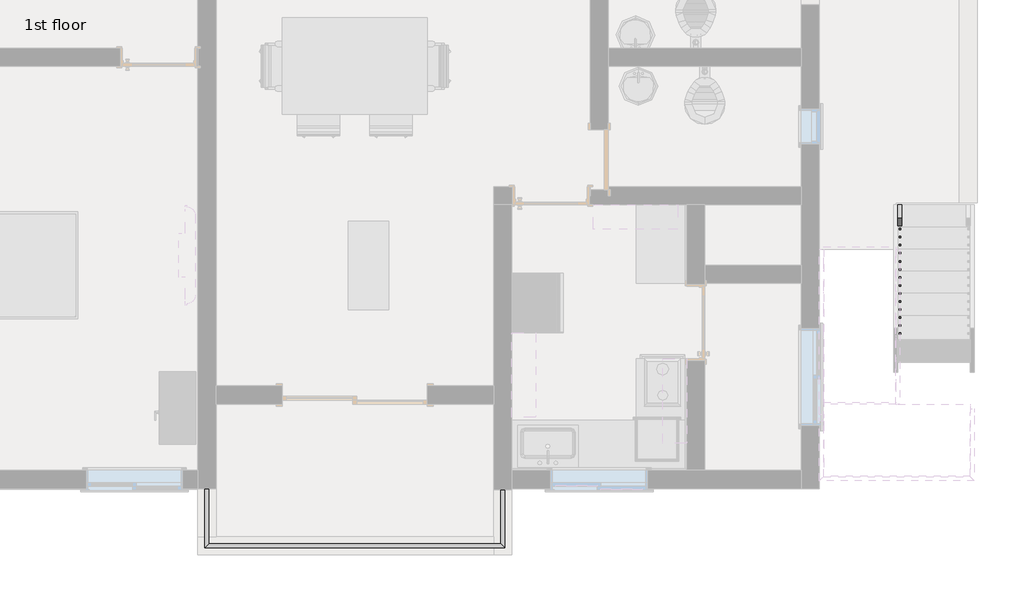
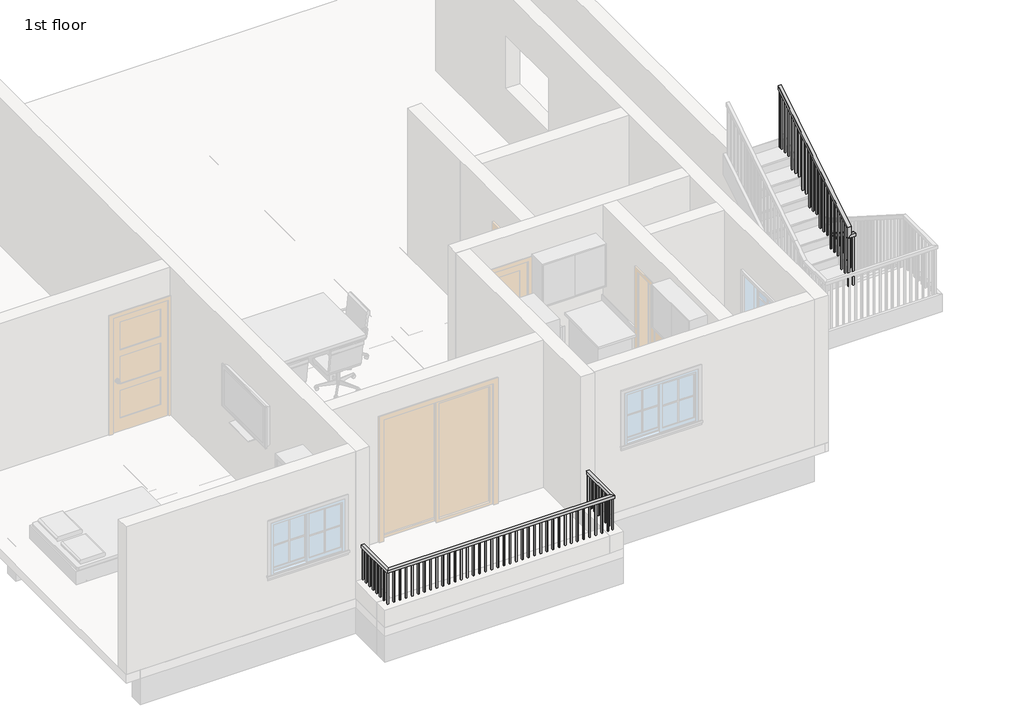
# One storey, part 4 of 8: 2 railings.
"""IFC4 building model written with IfcOpenShell, lengths in millimetres."""

from ifc_helpers import new_model, si_unit, frame, origin, place, context, project, spatial, polyline, outline, extrude, faceted_brep, element, save

model = new_model("IFC4")

# Units and contexts
model_context = context("Model", 3, world=origin())
ifc_project = project(units=[si_unit("LENGTHUNIT", "METRE", prefix="MILLI")], contexts=[model_context])

# Site, building, storey
site = spatial("IfcSite", under=ifc_project)
building = spatial("IfcBuilding", under=site)
storey = spatial("IfcBuildingStorey", under=building, Name="1st floor", Elevation=3810.0)

# Railings
placement = place(None, origin())
element("IfcRailing", 1, ObjectType="Handrail - Rectangular", at=placement, inside=storey, context=model_context, shape_type="SolidModel", body=[
    faceted_brep([(-12350.8993763, -4611.6564015, 4724.4), (-12350.8993763, -4611.6564015, 4673.6), (-12401.6993763, -4611.6564015, 4673.6), (-12401.6993763, -4611.6564015, 4724.4), (-12350.8993763, -5303.8064015, 4724.4), (-12350.8993763, -5303.8064015, 4673.6), (-12401.6993763, -5354.6064015, 4673.6), (-12401.6993763, -5354.6064015, 4724.4), (-8667.8993763, -5303.8064015, 4724.4), (-8667.8993763, -5303.8064015, 4673.6), (-8617.0993763, -5354.6064015, 4673.6), (-8617.0993763, -5354.6064015, 4724.4), (-8667.8993763, -4618.0064015, 4724.4), (-8617.0993763, -4618.0064015, 4724.4), (-8617.0993763, -4618.0064015, 4673.6), (-8667.8993763, -4618.0064015, 4673.6)], [[[0, 1, 2, 3]], [[1, 0, 4, 5]], [[2, 1, 5, 6]], [[3, 2, 6, 7]], [[0, 3, 7, 4]], [[5, 4, 8, 9]], [[6, 5, 9, 10]], [[7, 6, 10, 11]], [[4, 7, 11, 8]], [[12, 13, 14, 15]], [[9, 8, 12, 15]], [[10, 9, 15, 14]], [[11, 10, 14, 13]], [[8, 11, 13, 12]]]),
    extrude(outline(polyline([(-8632.9743763, -4729.1314015), (-8652.0243763, -4729.1314015), (-8652.0243763, -4710.0814015), (-8632.9743763, -4710.0814015), (-8632.9743763, -4729.1314015)])), frame((0.0, 0.0, 3810.0), z_axis=(0.0, 0.0, 1.0), x_axis=(1.0, 0.0, 0.0)), (0.0, 0.0, 1.0), 863.6),
    extrude(outline(polyline([(-8632.9743763, -4830.7314015), (-8652.0243763, -4830.7314015), (-8652.0243763, -4811.6814015), (-8632.9743763, -4811.6814015), (-8632.9743763, -4830.7314015)])), frame((0.0, 0.0, 3810.0), z_axis=(0.0, 0.0, 1.0), x_axis=(1.0, 0.0, 0.0)), (0.0, 0.0, 1.0), 863.6),
    extrude(outline(polyline([(-8632.9743763, -4932.3314015), (-8652.0243763, -4932.3314015), (-8652.0243763, -4913.2814015), (-8632.9743763, -4913.2814015), (-8632.9743763, -4932.3314015)])), frame((0.0, 0.0, 3810.0), z_axis=(0.0, 0.0, 1.0), x_axis=(1.0, 0.0, 0.0)), (0.0, 0.0, 1.0), 863.6),
    extrude(outline(polyline([(-8632.9743763, -5033.9314015), (-8652.0243763, -5033.9314015), (-8652.0243763, -5014.8814015), (-8632.9743763, -5014.8814015), (-8632.9743763, -5033.9314015)])), frame((0.0, 0.0, 3810.0), z_axis=(0.0, 0.0, 1.0), x_axis=(1.0, 0.0, 0.0)), (0.0, 0.0, 1.0), 863.6),
    extrude(outline(polyline([(-8632.9743763, -5135.5314015), (-8652.0243763, -5135.5314015), (-8652.0243763, -5116.4814015), (-8632.9743763, -5116.4814015), (-8632.9743763, -5135.5314015)])), frame((0.0, 0.0, 3810.0), z_axis=(0.0, 0.0, 1.0), x_axis=(1.0, 0.0, 0.0)), (0.0, 0.0, 1.0), 863.6),
    extrude(outline(polyline([(-8632.9743763, -5237.1314015), (-8652.0243763, -5237.1314015), (-8652.0243763, -5218.0814015), (-8632.9743763, -5218.0814015), (-8632.9743763, -5237.1314015)])), frame((0.0, 0.0, 3810.0), z_axis=(0.0, 0.0, 1.0), x_axis=(1.0, 0.0, 0.0)), (0.0, 0.0, 1.0), 863.6),
    extrude(outline(polyline([(-8728.2243763, -5338.7314015), (-8728.2243763, -5319.6814015), (-8709.1743763, -5319.6814015), (-8709.1743763, -5338.7314015), (-8728.2243763, -5338.7314015)])), frame((0.0, 0.0, 3810.0), z_axis=(0.0, 0.0, 1.0), x_axis=(1.0, 0.0, 0.0)), (0.0, 0.0, 1.0), 863.6),
    extrude(outline(polyline([(-8829.8243763, -5338.7314015), (-8829.8243763, -5319.6814015), (-8810.7743763, -5319.6814015), (-8810.7743763, -5338.7314015), (-8829.8243763, -5338.7314015)])), frame((0.0, 0.0, 3810.0), z_axis=(0.0, 0.0, 1.0), x_axis=(1.0, 0.0, 0.0)), (0.0, 0.0, 1.0), 863.6),
    extrude(outline(polyline([(-8931.4243763, -5338.7314015), (-8931.4243763, -5319.6814015), (-8912.3743763, -5319.6814015), (-8912.3743763, -5338.7314015), (-8931.4243763, -5338.7314015)])), frame((0.0, 0.0, 3810.0), z_axis=(0.0, 0.0, 1.0), x_axis=(1.0, 0.0, 0.0)), (0.0, 0.0, 1.0), 863.6),
    extrude(outline(polyline([(-9033.0243763, -5338.7314015), (-9033.0243763, -5319.6814015), (-9013.9743763, -5319.6814015), (-9013.9743763, -5338.7314015), (-9033.0243763, -5338.7314015)])), frame((0.0, 0.0, 3810.0), z_axis=(0.0, 0.0, 1.0), x_axis=(1.0, 0.0, 0.0)), (0.0, 0.0, 1.0), 863.6),
    extrude(outline(polyline([(-9134.6243763, -5338.7314015), (-9134.6243763, -5319.6814015), (-9115.5743763, -5319.6814015), (-9115.5743763, -5338.7314015), (-9134.6243763, -5338.7314015)])), frame((0.0, 0.0, 3810.0), z_axis=(0.0, 0.0, 1.0), x_axis=(1.0, 0.0, 0.0)), (0.0, 0.0, 1.0), 863.6),
    extrude(outline(polyline([(-9236.2243763, -5338.7314015), (-9236.2243763, -5319.6814015), (-9217.1743763, -5319.6814015), (-9217.1743763, -5338.7314015), (-9236.2243763, -5338.7314015)])), frame((0.0, 0.0, 3810.0), z_axis=(0.0, 0.0, 1.0), x_axis=(1.0, 0.0, 0.0)), (0.0, 0.0, 1.0), 863.6),
    extrude(outline(polyline([(-9337.8243763, -5338.7314015), (-9337.8243763, -5319.6814015), (-9318.7743763, -5319.6814015), (-9318.7743763, -5338.7314015), (-9337.8243763, -5338.7314015)])), frame((0.0, 0.0, 3810.0), z_axis=(0.0, 0.0, 1.0), x_axis=(1.0, 0.0, 0.0)), (0.0, 0.0, 1.0), 863.6),
    extrude(outline(polyline([(-9439.4243763, -5338.7314015), (-9439.4243763, -5319.6814015), (-9420.3743763, -5319.6814015), (-9420.3743763, -5338.7314015), (-9439.4243763, -5338.7314015)])), frame((0.0, 0.0, 3810.0), z_axis=(0.0, 0.0, 1.0), x_axis=(1.0, 0.0, 0.0)), (0.0, 0.0, 1.0), 863.6),
    extrude(outline(polyline([(-9541.0243763, -5338.7314015), (-9541.0243763, -5319.6814015), (-9521.9743763, -5319.6814015), (-9521.9743763, -5338.7314015), (-9541.0243763, -5338.7314015)])), frame((0.0, 0.0, 3810.0), z_axis=(0.0, 0.0, 1.0), x_axis=(1.0, 0.0, 0.0)), (0.0, 0.0, 1.0), 863.6),
    extrude(outline(polyline([(-9642.6243763, -5338.7314015), (-9642.6243763, -5319.6814015), (-9623.5743763, -5319.6814015), (-9623.5743763, -5338.7314015), (-9642.6243763, -5338.7314015)])), frame((0.0, 0.0, 3810.0), z_axis=(0.0, 0.0, 1.0), x_axis=(1.0, 0.0, 0.0)), (0.0, 0.0, 1.0), 863.6),
    extrude(outline(polyline([(-9744.2243763, -5338.7314015), (-9744.2243763, -5319.6814015), (-9725.1743763, -5319.6814015), (-9725.1743763, -5338.7314015), (-9744.2243763, -5338.7314015)])), frame((0.0, 0.0, 3810.0), z_axis=(0.0, 0.0, 1.0), x_axis=(1.0, 0.0, 0.0)), (0.0, 0.0, 1.0), 863.6),
    extrude(outline(polyline([(-9845.8243763, -5338.7314015), (-9845.8243763, -5319.6814015), (-9826.7743763, -5319.6814015), (-9826.7743763, -5338.7314015), (-9845.8243763, -5338.7314015)])), frame((0.0, 0.0, 3810.0), z_axis=(0.0, 0.0, 1.0), x_axis=(1.0, 0.0, 0.0)), (0.0, 0.0, 1.0), 863.6),
    extrude(outline(polyline([(-9947.4243763, -5338.7314015), (-9947.4243763, -5319.6814015), (-9928.3743763, -5319.6814015), (-9928.3743763, -5338.7314015), (-9947.4243763, -5338.7314015)])), frame((0.0, 0.0, 3810.0), z_axis=(0.0, 0.0, 1.0), x_axis=(1.0, 0.0, 0.0)), (0.0, 0.0, 1.0), 863.6),
    extrude(outline(polyline([(-10049.0243763, -5338.7314015), (-10049.0243763, -5319.6814015), (-10029.9743763, -5319.6814015), (-10029.9743763, -5338.7314015), (-10049.0243763, -5338.7314015)])), frame((0.0, 0.0, 3810.0), z_axis=(0.0, 0.0, 1.0), x_axis=(1.0, 0.0, 0.0)), (0.0, 0.0, 1.0), 863.6),
    extrude(outline(polyline([(-10150.6243763, -5338.7314015), (-10150.6243763, -5319.6814015), (-10131.5743763, -5319.6814015), (-10131.5743763, -5338.7314015), (-10150.6243763, -5338.7314015)])), frame((0.0, 0.0, 3810.0), z_axis=(0.0, 0.0, 1.0), x_axis=(1.0, 0.0, 0.0)), (0.0, 0.0, 1.0), 863.6),
    extrude(outline(polyline([(-10252.2243763, -5338.7314015), (-10252.2243763, -5319.6814015), (-10233.1743763, -5319.6814015), (-10233.1743763, -5338.7314015), (-10252.2243763, -5338.7314015)])), frame((0.0, 0.0, 3810.0), z_axis=(0.0, 0.0, 1.0), x_axis=(1.0, 0.0, 0.0)), (0.0, 0.0, 1.0), 863.6),
    extrude(outline(polyline([(-10353.8243763, -5338.7314015), (-10353.8243763, -5319.6814015), (-10334.7743763, -5319.6814015), (-10334.7743763, -5338.7314015), (-10353.8243763, -5338.7314015)])), frame((0.0, 0.0, 3810.0), z_axis=(0.0, 0.0, 1.0), x_axis=(1.0, 0.0, 0.0)), (0.0, 0.0, 1.0), 863.6),
    extrude(outline(polyline([(-10455.4243763, -5338.7314015), (-10455.4243763, -5319.6814015), (-10436.3743763, -5319.6814015), (-10436.3743763, -5338.7314015), (-10455.4243763, -5338.7314015)])), frame((0.0, 0.0, 3810.0), z_axis=(0.0, 0.0, 1.0), x_axis=(1.0, 0.0, 0.0)), (0.0, 0.0, 1.0), 863.6),
    extrude(outline(polyline([(-10557.0243763, -5338.7314015), (-10557.0243763, -5319.6814015), (-10537.9743763, -5319.6814015), (-10537.9743763, -5338.7314015), (-10557.0243763, -5338.7314015)])), frame((0.0, 0.0, 3810.0), z_axis=(0.0, 0.0, 1.0), x_axis=(1.0, 0.0, 0.0)), (0.0, 0.0, 1.0), 863.6),
    extrude(outline(polyline([(-10658.6243763, -5338.7314015), (-10658.6243763, -5319.6814015), (-10639.5743763, -5319.6814015), (-10639.5743763, -5338.7314015), (-10658.6243763, -5338.7314015)])), frame((0.0, 0.0, 3810.0), z_axis=(0.0, 0.0, 1.0), x_axis=(1.0, 0.0, 0.0)), (0.0, 0.0, 1.0), 863.6),
    extrude(outline(polyline([(-10760.2243763, -5338.7314015), (-10760.2243763, -5319.6814015), (-10741.1743763, -5319.6814015), (-10741.1743763, -5338.7314015), (-10760.2243763, -5338.7314015)])), frame((0.0, 0.0, 3810.0), z_axis=(0.0, 0.0, 1.0), x_axis=(1.0, 0.0, 0.0)), (0.0, 0.0, 1.0), 863.6),
    extrude(outline(polyline([(-10861.8243763, -5338.7314015), (-10861.8243763, -5319.6814015), (-10842.7743763, -5319.6814015), (-10842.7743763, -5338.7314015), (-10861.8243763, -5338.7314015)])), frame((0.0, 0.0, 3810.0), z_axis=(0.0, 0.0, 1.0), x_axis=(1.0, 0.0, 0.0)), (0.0, 0.0, 1.0), 863.6),
    extrude(outline(polyline([(-10963.4243763, -5338.7314015), (-10963.4243763, -5319.6814015), (-10944.3743763, -5319.6814015), (-10944.3743763, -5338.7314015), (-10963.4243763, -5338.7314015)])), frame((0.0, 0.0, 3810.0), z_axis=(0.0, 0.0, 1.0), x_axis=(1.0, 0.0, 0.0)), (0.0, 0.0, 1.0), 863.6),
    extrude(outline(polyline([(-11065.0243763, -5338.7314015), (-11065.0243763, -5319.6814015), (-11045.9743763, -5319.6814015), (-11045.9743763, -5338.7314015), (-11065.0243763, -5338.7314015)])), frame((0.0, 0.0, 3810.0), z_axis=(0.0, 0.0, 1.0), x_axis=(1.0, 0.0, 0.0)), (0.0, 0.0, 1.0), 863.6),
    extrude(outline(polyline([(-11166.6243763, -5338.7314015), (-11166.6243763, -5319.6814015), (-11147.5743763, -5319.6814015), (-11147.5743763, -5338.7314015), (-11166.6243763, -5338.7314015)])), frame((0.0, 0.0, 3810.0), z_axis=(0.0, 0.0, 1.0), x_axis=(1.0, 0.0, 0.0)), (0.0, 0.0, 1.0), 863.6),
    extrude(outline(polyline([(-11268.2243763, -5338.7314015), (-11268.2243763, -5319.6814015), (-11249.1743763, -5319.6814015), (-11249.1743763, -5338.7314015), (-11268.2243763, -5338.7314015)])), frame((0.0, 0.0, 3810.0), z_axis=(0.0, 0.0, 1.0), x_axis=(1.0, 0.0, 0.0)), (0.0, 0.0, 1.0), 863.6),
    extrude(outline(polyline([(-11369.8243763, -5338.7314015), (-11369.8243763, -5319.6814015), (-11350.7743763, -5319.6814015), (-11350.7743763, -5338.7314015), (-11369.8243763, -5338.7314015)])), frame((0.0, 0.0, 3810.0), z_axis=(0.0, 0.0, 1.0), x_axis=(1.0, 0.0, 0.0)), (0.0, 0.0, 1.0), 863.6),
    extrude(outline(polyline([(-11471.4243763, -5338.7314015), (-11471.4243763, -5319.6814015), (-11452.3743763, -5319.6814015), (-11452.3743763, -5338.7314015), (-11471.4243763, -5338.7314015)])), frame((0.0, 0.0, 3810.0), z_axis=(0.0, 0.0, 1.0), x_axis=(1.0, 0.0, 0.0)), (0.0, 0.0, 1.0), 863.6),
    extrude(outline(polyline([(-11573.0243763, -5338.7314015), (-11573.0243763, -5319.6814015), (-11553.9743763, -5319.6814015), (-11553.9743763, -5338.7314015), (-11573.0243763, -5338.7314015)])), frame((0.0, 0.0, 3810.0), z_axis=(0.0, 0.0, 1.0), x_axis=(1.0, 0.0, 0.0)), (0.0, 0.0, 1.0), 863.6),
    extrude(outline(polyline([(-11674.6243763, -5338.7314015), (-11674.6243763, -5319.6814015), (-11655.5743763, -5319.6814015), (-11655.5743763, -5338.7314015), (-11674.6243763, -5338.7314015)])), frame((0.0, 0.0, 3810.0), z_axis=(0.0, 0.0, 1.0), x_axis=(1.0, 0.0, 0.0)), (0.0, 0.0, 1.0), 863.6),
    extrude(outline(polyline([(-11776.2243763, -5338.7314015), (-11776.2243763, -5319.6814015), (-11757.1743763, -5319.6814015), (-11757.1743763, -5338.7314015), (-11776.2243763, -5338.7314015)])), frame((0.0, 0.0, 3810.0), z_axis=(0.0, 0.0, 1.0), x_axis=(1.0, 0.0, 0.0)), (0.0, 0.0, 1.0), 863.6),
    extrude(outline(polyline([(-11877.8243763, -5338.7314015), (-11877.8243763, -5319.6814015), (-11858.7743763, -5319.6814015), (-11858.7743763, -5338.7314015), (-11877.8243763, -5338.7314015)])), frame((0.0, 0.0, 3810.0), z_axis=(0.0, 0.0, 1.0), x_axis=(1.0, 0.0, 0.0)), (0.0, 0.0, 1.0), 863.6),
    extrude(outline(polyline([(-11979.4243763, -5338.7314015), (-11979.4243763, -5319.6814015), (-11960.3743763, -5319.6814015), (-11960.3743763, -5338.7314015), (-11979.4243763, -5338.7314015)])), frame((0.0, 0.0, 3810.0), z_axis=(0.0, 0.0, 1.0), x_axis=(1.0, 0.0, 0.0)), (0.0, 0.0, 1.0), 863.6),
    extrude(outline(polyline([(-12081.0243763, -5338.7314015), (-12081.0243763, -5319.6814015), (-12061.9743763, -5319.6814015), (-12061.9743763, -5338.7314015), (-12081.0243763, -5338.7314015)])), frame((0.0, 0.0, 3810.0), z_axis=(0.0, 0.0, 1.0), x_axis=(1.0, 0.0, 0.0)), (0.0, 0.0, 1.0), 863.6),
    extrude(outline(polyline([(-12182.6243763, -5338.7314015), (-12182.6243763, -5319.6814015), (-12163.5743763, -5319.6814015), (-12163.5743763, -5338.7314015), (-12182.6243763, -5338.7314015)])), frame((0.0, 0.0, 3810.0), z_axis=(0.0, 0.0, 1.0), x_axis=(1.0, 0.0, 0.0)), (0.0, 0.0, 1.0), 863.6),
    extrude(outline(polyline([(-12284.2243763, -5338.7314015), (-12284.2243763, -5319.6814015), (-12265.1743763, -5319.6814015), (-12265.1743763, -5338.7314015), (-12284.2243763, -5338.7314015)])), frame((0.0, 0.0, 3810.0), z_axis=(0.0, 0.0, 1.0), x_axis=(1.0, 0.0, 0.0)), (0.0, 0.0, 1.0), 863.6),
    extrude(outline(polyline([(-12385.8243763, -5313.3314015), (-12366.7743763, -5313.3314015), (-12366.7743763, -5332.3814015), (-12385.8243763, -5332.3814015), (-12385.8243763, -5313.3314015)])), frame((0.0, 0.0, 3810.0), z_axis=(0.0, 0.0, 1.0), x_axis=(1.0, 0.0, 0.0)), (0.0, 0.0, 1.0), 863.6),
    extrude(outline(polyline([(-12385.8243763, -5211.7314015), (-12366.7743763, -5211.7314015), (-12366.7743763, -5230.7814015), (-12385.8243763, -5230.7814015), (-12385.8243763, -5211.7314015)])), frame((0.0, 0.0, 3810.0), z_axis=(0.0, 0.0, 1.0), x_axis=(1.0, 0.0, 0.0)), (0.0, 0.0, 1.0), 863.6),
    extrude(outline(polyline([(-12385.8243763, -5110.1314015), (-12366.7743763, -5110.1314015), (-12366.7743763, -5129.1814015), (-12385.8243763, -5129.1814015), (-12385.8243763, -5110.1314015)])), frame((0.0, 0.0, 3810.0), z_axis=(0.0, 0.0, 1.0), x_axis=(1.0, 0.0, 0.0)), (0.0, 0.0, 1.0), 863.6),
    extrude(outline(polyline([(-12385.8243763, -5008.5314015), (-12366.7743763, -5008.5314015), (-12366.7743763, -5027.5814015), (-12385.8243763, -5027.5814015), (-12385.8243763, -5008.5314015)])), frame((0.0, 0.0, 3810.0), z_axis=(0.0, 0.0, 1.0), x_axis=(1.0, 0.0, 0.0)), (0.0, 0.0, 1.0), 863.6),
    extrude(outline(polyline([(-12385.8243763, -4906.9314015), (-12366.7743763, -4906.9314015), (-12366.7743763, -4925.9814015), (-12385.8243763, -4925.9814015), (-12385.8243763, -4906.9314015)])), frame((0.0, 0.0, 3810.0), z_axis=(0.0, 0.0, 1.0), x_axis=(1.0, 0.0, 0.0)), (0.0, 0.0, 1.0), 863.6),
    extrude(outline(polyline([(-12385.8243763, -4805.3314015), (-12366.7743763, -4805.3314015), (-12366.7743763, -4824.3814015), (-12385.8243763, -4824.3814015), (-12385.8243763, -4805.3314015)])), frame((0.0, 0.0, 3810.0), z_axis=(0.0, 0.0, 1.0), x_axis=(1.0, 0.0, 0.0)), (0.0, 0.0, 1.0), 863.6),
    extrude(outline(polyline([(-12385.8243763, -4703.7314015), (-12366.7743763, -4703.7314015), (-12366.7743763, -4722.7814015), (-12385.8243763, -4722.7814015), (-12385.8243763, -4703.7314015)])), frame((0.0, 0.0, 3810.0), z_axis=(0.0, 0.0, 1.0), x_axis=(1.0, 0.0, 0.0)), (0.0, 0.0, 1.0), 863.6),
    extrude(outline(polyline([(-8652.0243763, -5338.7314015), (-8652.0243763, -5319.6814015), (-8632.9743763, -5319.6814015), (-8632.9743763, -5338.7314015), (-8652.0243763, -5338.7314015)])), frame((0.0, 0.0, 3810.0), z_axis=(0.0, 0.0, 1.0), x_axis=(1.0, 0.0, 0.0)), (0.0, 0.0, 1.0), 863.6),
    extrude(outline(polyline([(-12385.8243763, -5319.6814015), (-12366.7743763, -5319.6814015), (-12366.7743763, -5338.7314015), (-12385.8243763, -5338.7314015), (-12385.8243763, -5319.6814015)])), frame((0.0, 0.0, 3810.0), z_axis=(0.0, 0.0, 1.0), x_axis=(1.0, 0.0, 0.0)), (0.0, 0.0, 1.0), 863.6),
    extrude(outline(polyline([(-8632.9743763, -4637.0564015), (-8652.0243763, -4637.0564015), (-8652.0243763, -4618.0064015), (-8632.9743763, -4618.0064015), (-8632.9743763, -4637.0564015)])), frame((0.0, 0.0, 3810.0), z_axis=(0.0, 0.0, 1.0), x_axis=(1.0, 0.0, 0.0)), (0.0, 0.0, 1.0), 863.6),
    extrude(outline(polyline([(-12385.8243763, -4611.6564015), (-12366.7743763, -4611.6564015), (-12366.7743763, -4630.7064015), (-12385.8243763, -4630.7064015), (-12385.8243763, -4611.6564015)])), frame((0.0, 0.0, 3810.0), z_axis=(0.0, 0.0, 1.0), x_axis=(1.0, 0.0, 0.0)), (0.0, 0.0, 1.0), 863.6),
])
element("IfcRailing", 2, ObjectType="Handrail - Rectangular", at=placement, inside=storey, context=model_context, shape_type="SolidModel", body=[
    faceted_brep([(-3600.5993763, -1023.9064015, 4902.2), (-3600.5993763, -1023.9064015, 4841.986276), (-3651.3993763, -1023.9064015, 4841.986276), (-3651.3993763, -1023.9064015, 4902.2), (-3600.5993763, -3538.5064015, 6502.4), (-3651.3993763, -3538.5064015, 6502.4), (-3651.3993763, -3538.5064015, 6442.186276), (-3600.5993763, -3538.5064015, 6442.186276)], [[[0, 1, 2, 3]], [[4, 5, 6, 7]], [[1, 0, 4, 7]], [[2, 1, 7, 6]], [[3, 2, 6, 5]], [[0, 3, 5, 4]]]),
    faceted_brep([(-3600.5993763, -3589.3064015, 6502.4), (-3600.5993763, -3589.3064015, 6451.6), (-3600.5993763, -3538.5064015, 6451.6), (-3600.5993763, -3538.5064015, 6502.4), (-3676.7993763, -3589.3064015, 6502.4), (-3676.7993763, -3538.5064015, 6502.4), (-3727.5993763, -3538.5064015, 6451.6), (-3727.5993763, -3589.3064015, 6451.6)], [[[0, 1, 2, 3]], [[4, 5, 6, 7]], [[1, 0, 4, 7]], [[2, 1, 7, 6]], [[3, 2, 6, 5]], [[0, 3, 5, 4]]]),
    faceted_brep([(-3676.7993763, -3589.3064015, 6502.4), (-3727.5993763, -3589.3064015, 6451.6), (-3727.5993763, -3538.5064015, 6451.6), (-3676.7993763, -3538.5064015, 6502.4), (-3676.7993763, -3589.3064015, 6647.8727273), (-3676.7993763, -3538.5064015, 6619.986276), (-3727.5993763, -3538.5064015, 6619.986276), (-3727.5993763, -3589.3064015, 6647.8727273)], [[[0, 1, 2, 3]], [[4, 5, 6, 7]], [[1, 0, 4, 7]], [[2, 1, 7, 6]], [[3, 2, 6, 5]], [[0, 3, 5, 4]]]),
    faceted_brep([(-3727.5993763, -3589.3064015, 6647.8727273), (-3727.5993763, -3538.5064015, 6619.986276), (-3676.7993763, -3538.5064015, 6619.986276), (-3676.7993763, -3589.3064015, 6647.8727273), (-3727.5993763, -1582.7064015, 7924.8), (-3676.7993763, -1582.7064015, 7924.8), (-3676.7993763, -1582.7064015, 7864.586276), (-3727.5993763, -1582.7064015, 7864.586276)], [[[0, 1, 2, 3]], [[4, 5, 6, 7]], [[1, 0, 4, 7]], [[2, 1, 7, 6]], [[3, 2, 6, 5]], [[0, 3, 5, 4]]]),
    extrude(outline(polyline([(-1643.0314015, 7826.1976396), (-1623.9814015, 7838.3203669), (-1623.9814015, 6832.6), (-1643.0314015, 6832.6), (-1643.0314015, 7826.1976396)])), frame((-3711.7243763, 0.0, 0.0), z_axis=(1.0, 0.0, 0.0), x_axis=(0.0, 1.0, 0.0)), (0.0, 0.0, 1.0), 19.05),
    extrude(outline(polyline([(-1744.6314015, 7761.5430941), (-1725.5814015, 7773.6658214), (-1725.5814015, 6832.6), (-1744.6314015, 6832.6), (-1744.6314015, 7761.5430941)])), frame((-3711.7243763, 0.0, 0.0), z_axis=(1.0, 0.0, 0.0), x_axis=(0.0, 1.0, 0.0)), (0.0, 0.0, 1.0), 19.05),
    extrude(outline(polyline([(-1846.2314015, 7696.8885487), (-1827.1814015, 7709.011276), (-1827.1814015, 6832.6), (-1846.2314015, 6832.6), (-1846.2314015, 7696.8885487)])), frame((-3711.7243763, 0.0, 0.0), z_axis=(1.0, 0.0, 0.0), x_axis=(0.0, 1.0, 0.0)), (0.0, 0.0, 1.0), 19.05),
    extrude(outline(polyline([(-1947.8314015, 7632.2340032), (-1928.7814015, 7644.3567305), (-1928.7814015, 6654.8), (-1947.8314015, 6654.8), (-1947.8314015, 7632.2340032)])), frame((-3711.7243763, 0.0, 0.0), z_axis=(1.0, 0.0, 0.0), x_axis=(0.0, 1.0, 0.0)), (0.0, 0.0, 1.0), 19.05),
    extrude(outline(polyline([(-2049.4314015, 7567.5794578), (-2030.3814015, 7579.7021851), (-2030.3814015, 6654.8), (-2049.4314015, 6654.8), (-2049.4314015, 7567.5794578)])), frame((-3711.7243763, 0.0, 0.0), z_axis=(1.0, 0.0, 0.0), x_axis=(0.0, 1.0, 0.0)), (0.0, 0.0, 1.0), 19.05),
    extrude(outline(polyline([(-2151.0314015, 7502.9249123), (-2131.9814015, 7515.0476396), (-2131.9814015, 6654.8), (-2151.0314015, 6654.8), (-2151.0314015, 7502.9249123)])), frame((-3711.7243763, 0.0, 0.0), z_axis=(1.0, 0.0, 0.0), x_axis=(0.0, 1.0, 0.0)), (0.0, 0.0, 1.0), 19.05),
    extrude(outline(polyline([(-2252.6314015, 7438.2703669), (-2233.5814015, 7450.3930941), (-2233.5814015, 6477.0), (-2252.6314015, 6477.0), (-2252.6314015, 7438.2703669)])), frame((-3711.7243763, 0.0, 0.0), z_axis=(1.0, 0.0, 0.0), x_axis=(0.0, 1.0, 0.0)), (0.0, 0.0, 1.0), 19.05),
    extrude(outline(polyline([(-2354.2314015, 7373.6158214), (-2335.1814015, 7385.7385487), (-2335.1814015, 6477.0), (-2354.2314015, 6477.0), (-2354.2314015, 7373.6158214)])), frame((-3711.7243763, 0.0, 0.0), z_axis=(1.0, 0.0, 0.0), x_axis=(0.0, 1.0, 0.0)), (0.0, 0.0, 1.0), 19.05),
    extrude(outline(polyline([(-2455.8314015, 7308.961276), (-2436.7814015, 7321.0840032), (-2436.7814015, 6299.2), (-2455.8314015, 6299.2), (-2455.8314015, 7308.961276)])), frame((-3711.7243763, 0.0, 0.0), z_axis=(1.0, 0.0, 0.0), x_axis=(0.0, 1.0, 0.0)), (0.0, 0.0, 1.0), 19.05),
    extrude(outline(polyline([(-2557.4314015, 7244.3067305), (-2538.3814015, 7256.4294578), (-2538.3814015, 6299.2), (-2557.4314015, 6299.2), (-2557.4314015, 7244.3067305)])), frame((-3711.7243763, 0.0, 0.0), z_axis=(1.0, 0.0, 0.0), x_axis=(0.0, 1.0, 0.0)), (0.0, 0.0, 1.0), 19.05),
    extrude(outline(polyline([(-2659.0314015, 7179.6521851), (-2639.9814015, 7191.7749123), (-2639.9814015, 6299.2), (-2659.0314015, 6299.2), (-2659.0314015, 7179.6521851)])), frame((-3711.7243763, 0.0, 0.0), z_axis=(1.0, 0.0, 0.0), x_axis=(0.0, 1.0, 0.0)), (0.0, 0.0, 1.0), 19.05),
    extrude(outline(polyline([(-2760.6314015, 7114.9976396), (-2741.5814015, 7127.1203669), (-2741.5814015, 6121.4), (-2760.6314015, 6121.4), (-2760.6314015, 7114.9976396)])), frame((-3711.7243763, 0.0, 0.0), z_axis=(1.0, 0.0, 0.0), x_axis=(0.0, 1.0, 0.0)), (0.0, 0.0, 1.0), 19.05),
    extrude(outline(polyline([(-2862.2314015, 7050.3430941), (-2843.1814015, 7062.4658214), (-2843.1814015, 6121.4), (-2862.2314015, 6121.4), (-2862.2314015, 7050.3430941)])), frame((-3711.7243763, 0.0, 0.0), z_axis=(1.0, 0.0, 0.0), x_axis=(0.0, 1.0, 0.0)), (0.0, 0.0, 1.0), 19.05),
    extrude(outline(polyline([(-2963.8314015, 6985.6885487), (-2944.7814015, 6997.811276), (-2944.7814015, 6121.4), (-2963.8314015, 6121.4), (-2963.8314015, 6985.6885487)])), frame((-3711.7243763, 0.0, 0.0), z_axis=(1.0, 0.0, 0.0), x_axis=(0.0, 1.0, 0.0)), (0.0, 0.0, 1.0), 19.05),
    extrude(outline(polyline([(-3065.4314015, 6921.0340032), (-3046.3814015, 6933.1567305), (-3046.3814015, 5943.6), (-3065.4314015, 5943.6), (-3065.4314015, 6921.0340032)])), frame((-3711.7243763, 0.0, 0.0), z_axis=(1.0, 0.0, 0.0), x_axis=(0.0, 1.0, 0.0)), (0.0, 0.0, 1.0), 19.05),
    extrude(outline(polyline([(-3167.0314015, 6856.3794578), (-3147.9814015, 6868.5021851), (-3147.9814015, 5943.6), (-3167.0314015, 5943.6), (-3167.0314015, 6856.3794578)])), frame((-3711.7243763, 0.0, 0.0), z_axis=(1.0, 0.0, 0.0), x_axis=(0.0, 1.0, 0.0)), (0.0, 0.0, 1.0), 19.05),
    extrude(outline(polyline([(-3268.6314015, 6791.7249123), (-3249.5814015, 6803.8476396), (-3249.5814015, 5943.6), (-3268.6314015, 5943.6), (-3268.6314015, 6791.7249123)])), frame((-3711.7243763, 0.0, 0.0), z_axis=(1.0, 0.0, 0.0), x_axis=(0.0, 1.0, 0.0)), (0.0, 0.0, 1.0), 19.05),
    extrude(outline(polyline([(-3370.2314015, 6727.0703669), (-3351.1814015, 6739.1930941), (-3351.1814015, 5765.8), (-3370.2314015, 5765.8), (-3370.2314015, 6727.0703669)])), frame((-3711.7243763, 0.0, 0.0), z_axis=(1.0, 0.0, 0.0), x_axis=(0.0, 1.0, 0.0)), (0.0, 0.0, 1.0), 19.05),
    extrude(outline(polyline([(-3471.8314015, 6662.4158214), (-3452.7814015, 6674.5385487), (-3452.7814015, 5765.8), (-3471.8314015, 5765.8), (-3471.8314015, 6662.4158214)])), frame((-3711.7243763, 0.0, 0.0), z_axis=(1.0, 0.0, 0.0), x_axis=(0.0, 1.0, 0.0)), (0.0, 0.0, 1.0), 19.05),
    extrude(outline(polyline([(-3471.8314015, 6399.7567305), (-3452.7814015, 6387.6340032), (-3452.7814015, 5410.2), (-3471.8314015, 5410.2), (-3471.8314015, 6399.7567305)])), frame((-3635.5243763, 0.0, 0.0), z_axis=(1.0, 0.0, 0.0), x_axis=(0.0, 1.0, 0.0)), (0.0, 0.0, 1.0), 19.05),
    extrude(outline(polyline([(-3370.2314015, 6335.1021851), (-3351.1814015, 6322.9794578), (-3351.1814015, 5410.2), (-3370.2314015, 5410.2), (-3370.2314015, 6335.1021851)])), frame((-3635.5243763, 0.0, 0.0), z_axis=(1.0, 0.0, 0.0), x_axis=(0.0, 1.0, 0.0)), (0.0, 0.0, 1.0), 19.05),
    extrude(outline(polyline([(-3268.6314015, 6270.4476396), (-3249.5814015, 6258.3249123), (-3249.5814015, 5410.2), (-3268.6314015, 5410.2), (-3268.6314015, 6270.4476396)])), frame((-3635.5243763, 0.0, 0.0), z_axis=(1.0, 0.0, 0.0), x_axis=(0.0, 1.0, 0.0)), (0.0, 0.0, 1.0), 19.05),
    extrude(outline(polyline([(-3167.0314015, 6205.7930941), (-3147.9814015, 6193.6703669), (-3147.9814015, 5232.4), (-3167.0314015, 5232.4), (-3167.0314015, 6205.7930941)])), frame((-3635.5243763, 0.0, 0.0), z_axis=(1.0, 0.0, 0.0), x_axis=(0.0, 1.0, 0.0)), (0.0, 0.0, 1.0), 19.05),
    extrude(outline(polyline([(-3065.4314015, 6141.1385487), (-3046.3814015, 6129.0158214), (-3046.3814015, 5232.4), (-3065.4314015, 5232.4), (-3065.4314015, 6141.1385487)])), frame((-3635.5243763, 0.0, 0.0), z_axis=(1.0, 0.0, 0.0), x_axis=(0.0, 1.0, 0.0)), (0.0, 0.0, 1.0), 19.05),
    extrude(outline(polyline([(-2963.8314015, 6076.4840032), (-2944.7814015, 6064.361276), (-2944.7814015, 5054.6), (-2963.8314015, 5054.6), (-2963.8314015, 6076.4840032)])), frame((-3635.5243763, 0.0, 0.0), z_axis=(1.0, 0.0, 0.0), x_axis=(0.0, 1.0, 0.0)), (0.0, 0.0, 1.0), 19.05),
    extrude(outline(polyline([(-2862.2314015, 6011.8294578), (-2843.1814015, 5999.7067305), (-2843.1814015, 5054.6), (-2862.2314015, 5054.6), (-2862.2314015, 6011.8294578)])), frame((-3635.5243763, 0.0, 0.0), z_axis=(1.0, 0.0, 0.0), x_axis=(0.0, 1.0, 0.0)), (0.0, 0.0, 1.0), 19.05),
    extrude(outline(polyline([(-2760.6314015, 5947.1749123), (-2741.5814015, 5935.0521851), (-2741.5814015, 5054.6), (-2760.6314015, 5054.6), (-2760.6314015, 5947.1749123)])), frame((-3635.5243763, 0.0, 0.0), z_axis=(1.0, 0.0, 0.0), x_axis=(0.0, 1.0, 0.0)), (0.0, 0.0, 1.0), 19.05),
    extrude(outline(polyline([(-2659.0314015, 5882.5203669), (-2639.9814015, 5870.3976396), (-2639.9814015, 4876.8), (-2659.0314015, 4876.8), (-2659.0314015, 5882.5203669)])), frame((-3635.5243763, 0.0, 0.0), z_axis=(1.0, 0.0, 0.0), x_axis=(0.0, 1.0, 0.0)), (0.0, 0.0, 1.0), 19.05),
    extrude(outline(polyline([(-2557.4314015, 5817.8658214), (-2538.3814015, 5805.7430941), (-2538.3814015, 4876.8), (-2557.4314015, 4876.8), (-2557.4314015, 5817.8658214)])), frame((-3635.5243763, 0.0, 0.0), z_axis=(1.0, 0.0, 0.0), x_axis=(0.0, 1.0, 0.0)), (0.0, 0.0, 1.0), 19.05),
    extrude(outline(polyline([(-2455.8314015, 5753.211276), (-2436.7814015, 5741.0885487), (-2436.7814015, 4876.8), (-2455.8314015, 4876.8), (-2455.8314015, 5753.211276)])), frame((-3635.5243763, 0.0, 0.0), z_axis=(1.0, 0.0, 0.0), x_axis=(0.0, 1.0, 0.0)), (0.0, 0.0, 1.0), 19.05),
    extrude(outline(polyline([(-2354.2314015, 5688.5567305), (-2335.1814015, 5676.4340032), (-2335.1814015, 4699.0), (-2354.2314015, 4699.0), (-2354.2314015, 5688.5567305)])), frame((-3635.5243763, 0.0, 0.0), z_axis=(1.0, 0.0, 0.0), x_axis=(0.0, 1.0, 0.0)), (0.0, 0.0, 1.0), 19.05),
    extrude(outline(polyline([(-2252.6314015, 5623.9021851), (-2233.5814015, 5611.7794578), (-2233.5814015, 4699.0), (-2252.6314015, 4699.0), (-2252.6314015, 5623.9021851)])), frame((-3635.5243763, 0.0, 0.0), z_axis=(1.0, 0.0, 0.0), x_axis=(0.0, 1.0, 0.0)), (0.0, 0.0, 1.0), 19.05),
    extrude(outline(polyline([(-2151.0314015, 5559.2476396), (-2131.9814015, 5547.1249123), (-2131.9814015, 4699.0), (-2151.0314015, 4699.0), (-2151.0314015, 5559.2476396)])), frame((-3635.5243763, 0.0, 0.0), z_axis=(1.0, 0.0, 0.0), x_axis=(0.0, 1.0, 0.0)), (0.0, 0.0, 1.0), 19.05),
    extrude(outline(polyline([(-2049.4314015, 5494.5930941), (-2030.3814015, 5482.4703669), (-2030.3814015, 4521.2), (-2049.4314015, 4521.2), (-2049.4314015, 5494.5930941)])), frame((-3635.5243763, 0.0, 0.0), z_axis=(1.0, 0.0, 0.0), x_axis=(0.0, 1.0, 0.0)), (0.0, 0.0, 1.0), 19.05),
    extrude(outline(polyline([(-1947.8314015, 5429.9385487), (-1928.7814015, 5417.8158214), (-1928.7814015, 4521.2), (-1947.8314015, 4521.2), (-1947.8314015, 5429.9385487)])), frame((-3635.5243763, 0.0, 0.0), z_axis=(1.0, 0.0, 0.0), x_axis=(0.0, 1.0, 0.0)), (0.0, 0.0, 1.0), 19.05),
    extrude(outline(polyline([(-1846.2314015, 5365.2840032), (-1827.1814015, 5353.161276), (-1827.1814015, 4343.4), (-1846.2314015, 4343.4), (-1846.2314015, 5365.2840032)])), frame((-3635.5243763, 0.0, 0.0), z_axis=(1.0, 0.0, 0.0), x_axis=(0.0, 1.0, 0.0)), (0.0, 0.0, 1.0), 19.05),
    extrude(outline(polyline([(-1744.6314015, 5300.6294578), (-1725.5814015, 5288.5067305), (-1725.5814015, 4343.4), (-1744.6314015, 4343.4), (-1744.6314015, 5300.6294578)])), frame((-3635.5243763, 0.0, 0.0), z_axis=(1.0, 0.0, 0.0), x_axis=(0.0, 1.0, 0.0)), (0.0, 0.0, 1.0), 19.05),
    extrude(outline(polyline([(-1643.0314015, 5235.9749123), (-1623.9814015, 5223.8521851), (-1623.9814015, 4343.4), (-1643.0314015, 4343.4), (-1643.0314015, 5235.9749123)])), frame((-3635.5243763, 0.0, 0.0), z_axis=(1.0, 0.0, 0.0), x_axis=(0.0, 1.0, 0.0)), (0.0, 0.0, 1.0), 19.05),
    extrude(outline(polyline([(-1541.4314015, 5171.3203669), (-1522.3814015, 5159.1976396), (-1522.3814015, 4165.6), (-1541.4314015, 4165.6), (-1541.4314015, 5171.3203669)])), frame((-3635.5243763, 0.0, 0.0), z_axis=(1.0, 0.0, 0.0), x_axis=(0.0, 1.0, 0.0)), (0.0, 0.0, 1.0), 19.05),
    extrude(outline(polyline([(-1439.8314015, 5106.6658214), (-1420.7814015, 5094.5430941), (-1420.7814015, 4165.6), (-1439.8314015, 4165.6), (-1439.8314015, 5106.6658214)])), frame((-3635.5243763, 0.0, 0.0), z_axis=(1.0, 0.0, 0.0), x_axis=(0.0, 1.0, 0.0)), (0.0, 0.0, 1.0), 19.05),
    extrude(outline(polyline([(-1338.2314015, 5042.011276), (-1319.1814015, 5029.8885487), (-1319.1814015, 4165.6), (-1338.2314015, 4165.6), (-1338.2314015, 5042.011276)])), frame((-3635.5243763, 0.0, 0.0), z_axis=(1.0, 0.0, 0.0), x_axis=(0.0, 1.0, 0.0)), (0.0, 0.0, 1.0), 19.05),
    extrude(outline(polyline([(-1236.6314015, 4977.3567305), (-1217.5814015, 4965.2340032), (-1217.5814015, 3987.8), (-1236.6314015, 3987.8), (-1236.6314015, 4977.3567305)])), frame((-3635.5243763, 0.0, 0.0), z_axis=(1.0, 0.0, 0.0), x_axis=(0.0, 1.0, 0.0)), (0.0, 0.0, 1.0), 19.05),
    extrude(outline(polyline([(-1135.0314015, 4912.7021851), (-1115.9814015, 4900.5794578), (-1115.9814015, 3987.8), (-1135.0314015, 3987.8), (-1135.0314015, 4912.7021851)])), frame((-3635.5243763, 0.0, 0.0), z_axis=(1.0, 0.0, 0.0), x_axis=(0.0, 1.0, 0.0)), (0.0, 0.0, 1.0), 19.05),
    extrude(outline(polyline([(-3692.6743763, -3554.3814015), (-3692.6743763, -3573.4314015), (-3711.7243763, -3573.4314015), (-3711.7243763, -3554.3814015), (-3692.6743763, -3554.3814015)])), frame((0.0, 0.0, 5588.0), z_axis=(0.0, 0.0, 1.0), x_axis=(1.0, 0.0, 0.0)), (0.0, 0.0, 1.0), 863.6),
    extrude(outline(polyline([(-3573.4314015, 6464.411276), (-3554.3814015, 6452.2885487), (-3554.3814015, 5588.0), (-3573.4314015, 5588.0), (-3573.4314015, 6464.411276)])), frame((-3635.5243763, 0.0, 0.0), z_axis=(1.0, 0.0, 0.0), x_axis=(0.0, 1.0, 0.0)), (0.0, 0.0, 1.0), 19.05),
    extrude(outline(polyline([(-1601.7564015, 7852.4635487), (-1582.7064015, 7864.586276), (-1582.7064015, 6832.6), (-1601.7564015, 6832.6), (-1601.7564015, 7852.4635487)])), frame((-3711.7243763, 0.0, 0.0), z_axis=(1.0, 0.0, 0.0), x_axis=(0.0, 1.0, 0.0)), (0.0, 0.0, 1.0), 19.05),
    extrude(outline(polyline([(-1042.9564015, 4854.1090032), (-1023.9064015, 4841.986276), (-1023.9064015, 3987.8), (-1042.9564015, 3987.8), (-1042.9564015, 4854.1090032)])), frame((-3635.5243763, 0.0, 0.0), z_axis=(1.0, 0.0, 0.0), x_axis=(0.0, 1.0, 0.0)), (0.0, 0.0, 1.0), 19.05),
])

save(model, "model.ifc")

# Revit data of these elements
# Type "Handrail - Rectangular"
#   Assembly Code = "C2010400"
#   built-in parameter 1008612 = 0.0416667 (stored number, unit not read)
#   built-in parameter 1008611 = 0.0416667 (stored number, unit not read)
#   built-in parameter 1008609 = 0.333333 (stored number, unit not read)
#   built-in parameter 1008604 = 0.166667 (stored number, unit not read)
#   built-in parameter 1008603 = 0.166667 (stored number, unit not read)
#   Railing Height = 3' - 0"
#   built-in parameter 1008630 = 2
#   built-in parameter 1008610 = 2
#   built-in parameter 1008618 = Baluster - Square : 3/4"
# Elements 1, 2 (IfcRailing, "Handrail - Rectangular")
#   Phase Created = New Construction
